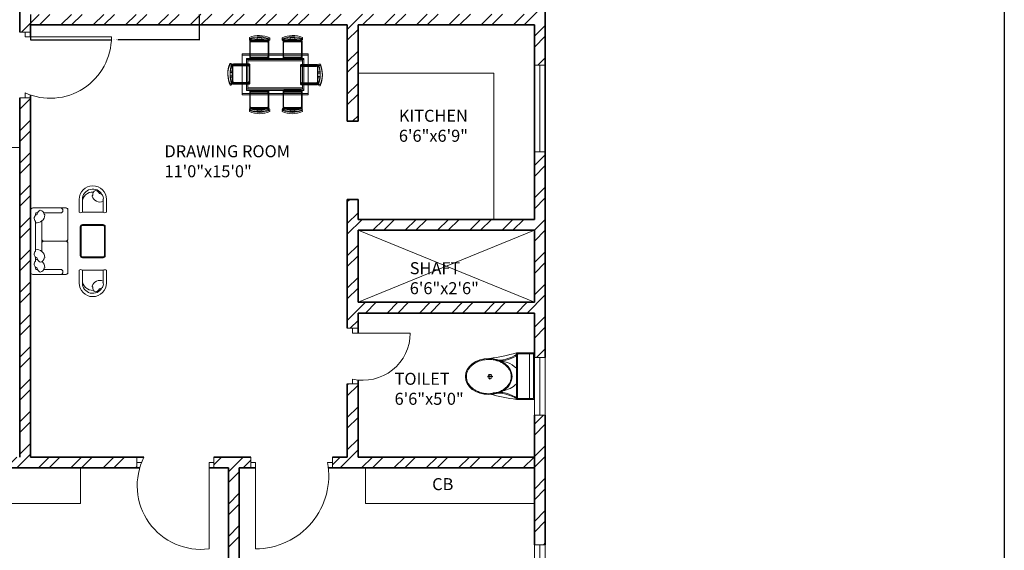
# Model space of a CAD drawing. Units: inches. Extents: x 2168 to 3056, y 1130 to 2629.
# Tile 6 of 42: x 2645 to 3056, y 1568 to 1789. Entities that reach past the tile are written whole.
import ezdxf

# ---------------------------------------------------------------- set-up
doc = ezdxf.new("R2010")
doc.units = ezdxf.units.IN
for name, color, linetype, lineweight in [('A-ANNO-DIMS', 2, 'Continuous', 18), ('A-ANNO-TEXT', 7, 'Continuous', 18), ('A-ANNO-TTLB', 7, 'Continuous', 25), ('A-AREA-IDEN', 7, 'Continuous', 18), ('A-DOOR', 21, 'Continuous', 18), ('A-FLOR-CASE', 71, 'Continuous', 18), ('A-FLOR-FIXT', 9, 'Continuous', 18), ('A-FLOR-OTLN', 7, 'Continuous', 18), ('A-FLOR-STRS', 71, 'Continuous', 18), ('A-FURN', 8, 'Continuous', 13), ('A-GLAZ', 201, 'Continuous', 18), ('A-WALL', 7, 'Continuous', 35)]:
    doc.layers.add(name, color=color, linetype=linetype, lineweight=lineweight)
doc.layers.add('A-WALL-PATT', color=143, linetype='Continuous', lineweight=13, true_color=0x7aafdf)
doc.styles.get("Standard").update_dxf_attribs({"font": 'arial.ttf'})
doc.dimstyles.get("Standard").update_dxf_attribs({"dimtxt": 0.18, "dimasz": 0.18, "dimexe": 0.18, "dimexo": 0.0625, "dimgap": 0.09, "dimtad": 0, "dimtih": 1, "dimtoh": 1, "dimdec": 4, "dimzin": 0, "dimdsep": 46, "dimtxsty": 'Standard', "dimcen": 0.09, "dimadec": 0, "dimazin": 0, "dimtfac": 1, "dimtdec": 4, "dimtofl": 0, "dimtmove": 0, "dimatfit": 3, "dimfxl": 1, "dimtolj": 1, "dimtzin": 0, "dimarcsym": 0})

# ---------------------------------------------------------------- blocks, each defined once
blk = doc.blocks.new('A$C31115884')
for p, q in [((283, 498), (223, 498)), ((258, 466), (258, 523)), ((0, 200), (0, 0)), ((520, 200), (0, 200)), ((10, 190), (10, 10)), ((510, 190), (10, 190)), ((510, 10), (510, 190)), ((520, 0), (520, 200)), ((510, 54), (0, 54)), ((10, 10), (510, 10)), ((0, 0), (520, 0))]:
    blk.add_line(p, q)
blk.add_circle((256, 496), 23.6)
for centre, radius, start, end in [((2778, -205), 2807, 165.4549, 171.7133), ((-295, 403), 365, 324.2091, 9.3499), ((-295, 403), 375, 324.2091, 9.3499), ((806, 403), 365, 170.6501, 215.7909), ((3237, 905), 2807, 188.2867, 194.5451), ((384, 406), 293, 190.2774, 224.1564), ((139, 406), 293, 315.8436, 2.6563), ((806, 403), 375, 179.2036, 215.7909)]:
    blk.add_arc(centre, radius, start, end)
blk.add_ellipse((256, 510), major_axis=(0, -261), ratio=0.772727)
blk.add_open_spline([(256, 259), (263, 259), (270, 260), (288, 262), (299, 265), (320, 273), (330, 278), (350, 291), (360, 299), (378, 316), (386, 326), (402, 347), (409, 358), (421, 383), (427, 395), (436, 422), (440, 436), (445, 465), (447, 480), (448, 509), (448, 524), (445, 553), (443, 568), (436, 596), (432, 610), (422, 636), (416, 649), (402, 672), (395, 683), (379, 703), (370, 712), (351, 728), (341, 735), (321, 746), (310, 751), (289, 757), (278, 759), (256, 761), (245, 761), (223, 757), (212, 754), (191, 746), (181, 741), (161, 728), (151, 720), (133, 703), (125, 693), (110, 672), (103, 660), (90, 636), (85, 623), (76, 596), (72, 582), (67, 553), (66, 538), (64, 509), (65, 494), (68, 465), (70, 450), (77, 422), (81, 408), (91, 382), (97, 370), (111, 346), (118, 335), (135, 316), (144, 307), (162, 291), (172, 284), (193, 273), (203, 269), (225, 262), (236, 260), (250, 259), (253, 259), (256, 259)], degree=3, knots=[0, 0, 0, 0, 0.110105, 0.110105, 0.285049, 0.285049, 0.459994, 0.459994, 0.634938, 0.634938, 0.809882, 0.809882, 0.984827, 0.984827, 1.159771, 1.159771, 1.334715, 1.334715, 1.50966, 1.50966, 1.684604, 1.684604, 1.859549, 1.859549, 2.034493, 2.034493, 2.209437, 2.209437, 2.384382, 2.384382, 2.559326, 2.559326, 2.73427, 2.73427, 2.909215, 2.909215, 3.084159, 3.084159, 3.259103, 3.259103, 3.434048, 3.434048, 3.608992, 3.608992, 3.783936, 3.783936, 3.958881, 3.958881, 4.133825, 4.133825, 4.30877, 4.30877, 4.483714, 4.483714, 4.658658, 4.658658, 4.833603, 4.833603, 5.008547, 5.008547, 5.183491, 5.183491, 5.358436, 5.358436, 5.53338, 5.53338, 5.708324, 5.708324, 5.883269, 5.883269, 6.058213, 6.058213, 6.233158, 6.233158, 6.283185, 6.283185, 6.283185, 6.283185])
blk = doc.blocks.new('A$C1352')
at = {"color": 0}
for points in [[(0.003, 0.053), (0.003, 0.553, -0.414214), (0.053, 0.603), (0.753, 0.603, -0.414214), (0.803, 0.553), (0.803, 0.053, -0.414214), (0.753, 0.003), (0.053, 0.003, -0.414214)], [(0.023, 0.053), (0.023, 0.553, -0.414214), (0.053, 0.583), (0.753, 0.583, -0.414214), (0.783, 0.553), (0.783, 0.053, -0.414214), (0.753, 0.023), (0.053, 0.023, -0.414214)]]:
    blk.add_lwpolyline(points, format="xyb", close=True, dxfattribs=at)
blk = doc.blocks.new('CHAIR-LOUNGE')
blk.add_line((10.04, 5.71), (10.04, 10.98))
at = {"ltscale": 0.03}
blk.add_lwpolyline([(10.04, 10.98, -0.369229), (11.42, 10.98), (11.42, 5.7, -1), (0, 5.72), (0, 10.99, -0.369229), (1.39, 10.99)], format="xyb", close=True, dxfattribs=at)
blk.add_lwpolyline([(9.55, 3.71, -0.785087), (1.38, 5.71), (1.39, 10.99)], format="xyb")
for centre, radius, start, end in [((5.71, 6.93), 4.33, 179.9461, 273.658), ((5.63, 4.23), 0.207, 150.6238, 293.7423), ((8.67, 3.43), 3.35, 67.0143, 164.2857), ((8.41, 5.02), 1.73, 272.9922, 34.1401), ((5.71, 5.71), 4.33, 358.8536, 359.9461), ((7.44, 3.63), 1.78, 166.6403, 249.4695), ((6.65, 3.91), 1.95, 274.9999, 341.3534)]:
    blk.add_arc(centre, radius, start, end)
blk = doc.blocks.new('TABLE-DINING')
for points in [[(0, 17.02), (27.45, 17.02), (27.45, 0.55), (0, 0.55)], [(0, 17.02), (27.45, 17.02), (27.45, 0.55), (0, 0.55)], [(0, 16.47), (27.45, 16.47), (27.45, 0), (0, 0)], [(0, 16.47), (27.45, 16.47), (27.45, 0), (0, 0)], [(1.83, 15.19), (25.62, 15.19), (25.62, 2.38), (1.83, 2.38)], [(1.83, 15.19), (25.62, 15.19), (25.62, 2.38), (1.83, 2.38)], [(1.83, 14.64), (25.62, 14.64), (25.62, 1.83), (1.83, 1.83)], [(1.83, 14.64), (25.62, 14.64), (25.62, 1.83), (1.83, 1.83)], [(2.38, 14.64), (25.07, 14.64), (25.07, 2.93), (2.38, 2.93)], [(2.38, 14.64), (25.07, 14.64), (25.07, 2.93), (2.38, 2.93)], [(2.38, 14.09), (25.07, 14.09), (25.07, 2.38), (2.38, 2.38)], [(2.38, 14.09), (25.07, 14.09), (25.07, 2.38), (2.38, 2.38)]]:
    blk.add_lwpolyline(points, close=True)
blk = doc.blocks.new('CUPBOARD-BEDROOM')
blk.add_lwpolyline([(0, 14.89), (70.36, 14.89), (70.36, 0), (0, 0)], close=True)
blk = doc.blocks.new('CHAIR-DINING-SIDE')
for points in [[(7.85, 2.38, 0.414214), (8.33, 2.86), (8.33, 9.24, 0.414214), (7.85, 9.73), (0.91, 9.73, 0.414214), (0.42, 9.24), (0.42, 2.86, 0.414214), (0.91, 2.38), (7.85, 2.38)], [(7.85, 2.38, 0.414214), (8.33, 2.86), (8.33, 9.24, 0.414214), (7.85, 9.73), (0.91, 9.73, 0.414214), (0.42, 9.24), (0.42, 2.86, 0.414214), (0.91, 2.38), (7.85, 2.38)], [(7.85, 1.83, 0.414214), (8.33, 2.31), (8.33, 8.69, 0.414214), (7.85, 9.18), (0.91, 9.18, 0.414214), (0.42, 8.69), (0.42, 2.31, 0.414214), (0.91, 1.83), (7.85, 1.83)], [(7.85, 1.83, 0.414214), (8.33, 2.31), (8.33, 8.69, 0.414214), (7.85, 9.18), (0.91, 9.18, 0.414214), (0.42, 8.69), (0.42, 2.31, 0.414214), (0.91, 1.83), (7.85, 1.83)], [(8.06, 2.08, -0.175809), (0.59, 2.13, 0.578392), (0.02, 1.51, 0.214524), (8.46, 1.4, 0.552014), (8.06, 2.08, -0.065079)], [(8.06, 2.08, -0.175809), (0.59, 2.13, 0.578392), (0.02, 1.51, 0.214524), (8.46, 1.4, 0.552014), (8.06, 2.08, -0.065079)], [(8.06, 1.53, -0.175809), (0.59, 1.58, 0.578392), (0.02, 0.96, 0.214524), (8.46, 0.85, 0.552014), (8.06, 1.53, -0.065079)], [(8.06, 1.53, -0.175809), (0.59, 1.58, 0.578392), (0.02, 0.96, 0.214524), (8.46, 0.85, 0.552014), (8.06, 1.53, -0.065079)], [(3.34, 2.38), (3.34, 1.5, -0.064759)], [(3.34, 2.38), (3.34, 1.5, -0.064759)], [(3.34, 1.83), (3.34, 0.95, -0.064759)], [(3.34, 1.83), (3.34, 0.95, -0.064759)]]:
    blk.add_lwpolyline(points, format="xyb")
for points in [[(7.84, 2.6), (1.13, 2.6, -0.414214), (0.64, 3.08), (0.64, 9.02, -0.414214), (1.13, 9.51), (7.84, 9.51, -0.512069), (8.11, 9.02), (8.11, 3.08, -0.512069)], [(7.84, 2.6), (1.13, 2.6, -0.414214), (0.64, 3.08), (0.64, 9.02, -0.414214), (1.13, 9.51), (7.84, 9.51, -0.512069), (8.11, 9.02), (8.11, 3.08, -0.512069)], [(7.84, 2.05), (1.13, 2.05, -0.414214), (0.64, 2.53), (0.64, 8.48, -0.414214), (1.13, 8.96), (7.84, 8.96, -0.512069), (8.11, 8.48), (8.11, 2.53, -0.512069)], [(7.84, 2.05), (1.13, 2.05, -0.414214), (0.64, 2.53), (0.64, 8.48, -0.414214), (1.13, 8.96), (7.84, 8.96, -0.512069), (8.11, 8.48), (8.11, 2.53, -0.512069)]]:
    blk.add_lwpolyline(points, format="xyb", close=True)
for points in [[(5.29, 1.48), (5.29, 2.38)], [(5.29, 1.48), (5.29, 2.38)], [(5.29, 0.93), (5.29, 1.83)], [(5.29, 0.93), (5.29, 1.83)]]:
    blk.add_lwpolyline(points)
blk = doc.blocks.new('CHAIR-DINING-END')
for points in [[(1.58, 1.14, -0.578392), (0.96, 0.57, -0.214524), (0.85, 9.01, -0.552014), (1.53, 8.61, 0.175809), (1.58, 1.14)], [(1.58, 1.14, -0.578392), (0.96, 0.57, -0.214524), (0.85, 9.01, -0.552014), (1.53, 8.61, 0.175809), (1.58, 1.14)], [(1.58, 0.59, -0.578392), (0.96, 0.02, -0.214524), (0.85, 8.46, -0.552014), (1.53, 8.06, 0.175809), (1.58, 0.59)], [(1.58, 0.59, -0.578392), (0.96, 0.02, -0.214524), (0.85, 8.46, -0.552014), (1.53, 8.06, 0.175809), (1.58, 0.59)], [(1.83, 8.39, -0.414214), (2.31, 8.88), (8.69, 8.88, -0.414214), (9.18, 8.39), (9.18, 1.45, -0.414214), (8.69, 0.97), (2.31, 0.97, -0.414214), (1.83, 1.45), (1.83, 8.39)], [(1.83, 8.39, -0.414214), (2.31, 8.88), (8.69, 8.88, -0.414214), (9.18, 8.39), (9.18, 1.45, -0.414214), (8.69, 0.97), (2.31, 0.97, -0.414214), (1.83, 1.45), (1.83, 8.39)], [(1.83, 7.85, -0.414214), (2.31, 8.33), (8.69, 8.33, -0.414214), (9.18, 7.85), (9.18, 0.91, -0.414214), (8.69, 0.42), (2.31, 0.42, -0.414214), (1.83, 0.91), (1.83, 7.85)], [(1.83, 7.85, -0.414214), (2.31, 8.33), (8.69, 8.33, -0.414214), (9.18, 7.85), (9.18, 0.91, -0.414214), (8.69, 0.42), (2.31, 0.42, -0.414214), (1.83, 0.91), (1.83, 7.85)], [(1.83, 3.89), (0.95, 3.89, 0.064759)], [(1.83, 3.89), (0.95, 3.89, 0.064759)], [(1.83, 3.34), (0.95, 3.34, 0.064759)], [(1.83, 3.34), (0.95, 3.34, 0.064759)]]:
    blk.add_lwpolyline(points, format="xyb")
for points in [[(2.05, 8.39), (2.05, 1.67, 0.414214), (2.53, 1.19), (8.48, 1.19, 0.414214), (8.96, 1.67), (8.96, 8.39, 0.512069), (8.48, 8.66), (2.53, 8.66, 0.512069)], [(2.05, 8.39), (2.05, 1.67, 0.414214), (2.53, 1.19), (8.48, 1.19, 0.414214), (8.96, 1.67), (8.96, 8.39, 0.512069), (8.48, 8.66), (2.53, 8.66, 0.512069)], [(2.05, 7.84), (2.05, 1.12, 0.414214), (2.53, 0.64), (8.48, 0.64, 0.414214), (8.96, 1.12), (8.96, 7.84, 0.512069), (8.48, 8.11), (2.53, 8.11, 0.512069)], [(2.05, 7.84), (2.05, 1.12, 0.414214), (2.53, 0.64), (8.48, 0.64, 0.414214), (8.96, 1.12), (8.96, 7.84, 0.512069), (8.48, 8.11), (2.53, 8.11, 0.512069)]]:
    blk.add_lwpolyline(points, format="xyb", close=True)
for points in [[(0.93, 5.84), (1.83, 5.84)], [(0.93, 5.83), (1.83, 5.83)], [(0.93, 5.29), (1.83, 5.29)], [(0.93, 5.29), (1.83, 5.29)]]:
    blk.add_lwpolyline(points)
blk = doc.blocks.new('WIN-24-OPPOSED-JAMBS')
for p, q in [((0, 4.5), (0, 0)), ((0, 4.5), (24, 4.5)), ((24, 2.25), (24, 4.5)), ((24, 4.5), (24, 0)), ((0, 0), (0, 2.25)), ((0, 2.25), (24, 2.25)), ((0, 0), (24, 0))]:
    blk.add_line(p, q)
blk = doc.blocks.new('WIN-60-OPPOSED-JAMBS')
for p, q in [((2.25, 60), (0, 60)), ((0, 60), (4.5, 60)), ((0, 60), (0, 0)), ((2.25, 0), (2.25, 60)), ((4.5, 60), (4.5, 0)), ((0, 0), (4.5, 0)), ((4.5, 0), (2.25, 0))]:
    blk.add_line(p, q)
blk = doc.blocks.new('*D18')
at = {"layer": 'A-ANNO-DIMS', "color": 0, "lineweight": -2, "transparency": 16777216}
for p, q in [((2649.8, 1791.2), (2649.8, 1780.53)), ((2720.15, 1791.2), (2720.15, 1780.53)), ((2649.98, 1780.71), (2683.7, 1780.71)), ((2719.97, 1780.71), (2686.25, 1780.71))]:
    blk.add_line(p, q, dxfattribs=at)
at = {"layer": 'A-ANNO-DIMS', "color": 0, "transparency": 16777216}
for points in [[(2649.98, 1780.74), (2649.98, 1780.68), (2649.8, 1780.71)], [(2719.97, 1780.74), (2719.97, 1780.68), (2720.15, 1780.71)]]:
    blk.add_solid(points, dxfattribs=at)
at = {"layer": 'Defpoints', "color": 0, "transparency": 16777216}
for p in [(2649.8, 1791.27), (2720.15, 1791.27), (2720.15, 1780.71)]:
    blk.add_point(p, dxfattribs=at)
at = {"layer": 'A-ANNO-DIMS', "color": 0, "transparency": 16777216, "insert": (2684.98, 1780.71), "char_height": 0.18, "attachment_point": 5}
blk.add_mtext('\\A1;CUPBOARD 70 TYP.', dxfattribs=at)

msp = doc.modelspace()

# ---------------------------------------------------------------- hatches: boundary and pattern name
at = {"layer": 'A-WALL-PATT'}
h = msp.add_hatch(dxfattribs=at)
h.set_pattern_fill('ANSI32', color=256)
h.paths.add_polyline_path([(2463.8, 2409.39), (2467.39, 2409.39), (2467.39, 2413.89), (2454.77, 2413.89), (2454.77, 2411.64), (2454.77, 2409.39), (2459.3, 2409.39), (2459.3, 2265.39), (2455.64, 2265.39), (2455.64, 2260.89), (2467.35, 2260.89), (2467.35, 2263.14), (2467.35, 2265.39), (2463.8, 2265.39)])
h.paths.add_polyline_path([(2431.6, 2413.89), (2409.65, 2413.89), (2409.65, 2409.39), (2431.6, 2409.39), (2431.6, 2411.64)])
h.paths.add_polyline_path([(2349.65, 2413.89), (2331.8, 2413.89), (2331.8, 2362.67), (2336.3, 2362.67), (2336.3, 2409.39), (2349.65, 2409.39), (2349.65, 2411.64)])
h.paths.add_polyline_path([(2634.15, 2411.64), (2634.15, 2413.89), (2562.29, 2413.89), (2562.29, 2409.39), (2595.8, 2409.39), (2595.8, 2280.31), (2595.83, 2280.31), (2595.83, 2265.39), (2499.91, 2265.39), (2499.91, 2260.89), (2550.8, 2260.89), (2550.8, 2117.31), (2555.3, 2117.31), (2555.3, 2168.08), (2571.93, 2168.08), (2571.93, 2176.89), (2559.8, 2176.89), (2559.8, 2256.39), (2640.8, 2256.39), (2640.8, 2176.89), (2626.43, 2176.89), (2626.43, 2168.08), (2645.3, 2168.08), (2645.3, 2116.64), (2649.8, 2116.64), (2649.8, 2260.89), (2691.25, 2260.89), (2691.25, 2263.14), (2691.25, 2265.39), (2670.65, 2265.39), (2670.65, 2265.36), (2600.3, 2265.36), (2600.3, 2280.26), (2600.3, 2409.39), (2634.15, 2409.39)])
h.paths.add_polyline_path([(2600.3, 2473.89), (2612.84, 2473.89), (2612.84, 2478.39), (2572.64, 2478.39), (2572.64, 2473.89), (2595.8, 2473.89), (2595.8, 2413.89), (2600.3, 2413.89)])
h.paths.add_polyline_path([(2535.8, 2473.89), (2548.64, 2473.89), (2548.64, 2478.39), (2531.4, 2478.39), (2531.4, 2413.89), (2521.6, 2413.89), (2521.6, 2409.39), (2539.24, 2409.39), (2539.24, 2411.64), (2539.24, 2413.89), (2535.8, 2413.89)])
h.paths.add_polyline_path([(2664.8, 2478.39), (2636.84, 2478.39), (2636.84, 2473.89), (2660.3, 2473.89), (2660.3, 2413.89), (2656.17, 2413.89), (2656.17, 2409.39), (2671.68, 2409.39), (2671.68, 2411.64), (2671.68, 2413.89), (2664.8, 2413.89)])
h.paths.add_polyline_path([(2705.94, 2413.89), (2695.68, 2413.89), (2695.68, 2409.39), (2705.94, 2409.39)])
h.paths.add_polyline_path([(2741.35, 2413.89), (2728.73, 2413.89), (2728.73, 2411.64), (2728.73, 2409.39), (2732.3, 2409.39), (2732.3, 2265.39), (2725.73, 2265.39), (2725.73, 2260.89), (2740.92, 2260.89), (2740.92, 2263.14), (2740.92, 2265.39), (2736.8, 2265.39), (2736.8, 2409.39), (2741.35, 2409.39)])
h.paths.add_polyline_path([(2785.65, 2413.89), (2764.55, 2413.89), (2764.49, 2409.39), (2785.65, 2409.39), (2785.65, 2411.64)])
h.paths.add_polyline_path([(2864.3, 2413.89), (2845.65, 2413.89), (2845.65, 2409.39), (2859.8, 2409.39), (2859.8, 2368.43), (2864.3, 2368.43)])
h.paths.add_polyline_path([(2864.3, 2308.43), (2862.05, 2308.43), (2859.8, 2308.43), (2859.8, 2265.39), (2774.48, 2265.39), (2774.48, 2263.14), (2774.48, 2260.89), (2781.8, 2260.89), (2781.8, 2226.65), (2786.3, 2226.65), (2786.3, 2260.89), (2859.8, 2260.89), (2859.8, 2241.35), (2864.3, 2241.35)])
h.paths.add_polyline_path([(2864.3, 2217.35), (2862.05, 2217.35), (2859.8, 2217.35), (2859.8, 2200.89), (2786.3, 2200.89), (2786.3, 2205.93), (2784.05, 2205.93), (2781.8, 2205.93), (2781.8, 2150.97), (2786.3, 2150.97), (2786.3, 2161.89), (2859.8, 2161.89), (2859.8, 2144.42), (2864.3, 2144.42)])
h.paths.add_polyline_path([(2859.8, 2196.39), (2859.8, 2166.39), (2786.3, 2166.39), (2786.3, 2196.39)], flags=16)
h.paths.add_polyline_path([(2864.3, 2108.42), (2862.05, 2108.42), (2859.8, 2108.42), (2859.8, 2080.89), (2786.3, 2080.89), (2786.3, 2111.99), (2781.8, 2111.99), (2781.8, 2080.89), (2649.8, 2080.89), (2649.8, 2086.04), (2647.55, 2086.04), (2645.3, 2086.04), (2645.3, 2071.74), (2649.8, 2071.74), (2649.8, 2076.39), (2781.8, 2076.39), (2781.8, 2041.79), (2786.3, 2041.79), (2786.3, 2076.39), (2859.8, 2076.39), (2859.8, 2058.58), (2864.3, 2058.58)])
h.paths.add_polyline_path([(2864.3, 2022.58), (2859.8, 2022.58), (2859.8, 1992.39), (2786.3, 1992.39), (2786.3, 1999.57), (2781.8, 1999.57), (2781.8, 1848.09), (2784.05, 1848.09), (2786.3, 1848.09), (2786.3, 1851.39), (2859.8, 1851.39), (2859.8, 1838.26), (2864.3, 1838.26)], flags=17)
h.paths.add_polyline_path([(2859.8, 1987.89), (2859.8, 1855.89), (2786.3, 1855.89), (2786.3, 1987.89)], flags=16)
h.paths.add_polyline_path([(2823.05, 1987.89), (2841.42, 1921.89), (2823.05, 1855.89)], flags=0)
h.paths.add_polyline_path([(2864.3, 1814.26), (2859.8, 1814.26), (2859.8, 1791.39), (2786.3, 1791.39), (2786.3, 1825.66), (2784.05, 1825.66), (2781.8, 1825.66), (2781.8, 1791.39), (2720.15, 1791.39), (2720.15, 1791.27), (2649.8, 1791.27), (2649.8, 1806.16), (2649.8, 2038.98), (2647.55, 2038.98), (2645.3, 2038.98), (2645.3, 1783.93), (2649.8, 1783.93), (2649.8, 1786.89), (2781.8, 1786.89), (2781.8, 1746.79), (2786.3, 1746.79), (2786.3, 1786.89), (2859.8, 1786.89), (2859.8, 1770.08), (2864.3, 1770.08)])
h.paths.add_polyline_path([(2864.3, 1734.08), (2862.05, 1734.08), (2859.8, 1734.08), (2859.8, 1705.89), (2786.3, 1705.89), (2786.3, 1714.17), (2781.8, 1714.17), (2781.8, 1660.53), (2786.3, 1660.53), (2786.3, 1666.89), (2859.8, 1666.89), (2859.8, 1648.34), (2864.3, 1648.34)])
h.paths.add_polyline_path([(2786.3, 1701.39), (2859.8, 1701.39), (2859.8, 1671.39), (2786.3, 1671.39)], flags=16)
h.paths.add_polyline_path([(2649.8, 1756.58), (2647.55, 1756.58), (2645.3, 1756.58), (2645.3, 1606.89), (2555.3, 1606.89), (2555.3, 1749.51), (2553.05, 1749.51), (2550.8, 1749.51), (2550.8, 1606.89), (2503.01, 1606.89), (2503.01, 1604.64), (2503.01, 1602.39), (2595.8, 1602.39), (2595.85, 1602.39), (2595.85, 1587.5), (2595.8, 1458.39), (2561.5, 1458.39), (2561.5, 1456.14), (2561.5, 1453.89), (2595.8, 1453.89), (2595.8, 1381.89), (2573.44, 1381.89), (2573.44, 1377.39), (2613.01, 1377.39), (2613.01, 1379.64), (2613.01, 1381.89), (2600.3, 1381.89), (2600.3, 1453.89), (2634.33, 1453.89), (2634.33, 1458.39), (2600.3, 1458.39), (2600.3, 1602.39), (2670.65, 1602.39), (2694.09, 1602.39), (2694.09, 1606.89), (2649.8, 1606.89)])
h.paths.add_polyline_path([(2736.8, 1602.39), (2741.56, 1602.39), (2741.56, 1606.89), (2726.2, 1606.89), (2726.2, 1604.64), (2726.2, 1602.39), (2732.3, 1602.39), (2732.3, 1458.39), (2727.9, 1458.39), (2727.9, 1453.89), (2740.82, 1453.89), (2740.82, 1456.14), (2740.82, 1458.39), (2736.8, 1458.39)])
h.paths.add_polyline_path([(2859.8, 1606.89), (2786.3, 1606.89), (2786.3, 1637.33), (2784.05, 1637.33), (2781.8, 1637.33), (2781.8, 1606.89), (2775.61, 1606.89), (2775.61, 1602.39), (2859.8, 1602.39)])
h.paths.add_polyline_path([(2864.3, 1624.34), (2862.05, 1624.34), (2859.8, 1624.34), (2859.8, 1570.39), (2864.3, 1570.39)])
h.paths.add_polyline_path([(2864.3, 1510.39), (2862.05, 1510.39), (2859.8, 1510.39), (2859.8, 1458.39), (2846.73, 1458.39), (2846.73, 1456.14), (2846.73, 1453.89), (2864.3, 1453.89)])
h.paths.add_polyline_path([(2786.73, 1458.39), (2765.44, 1458.39), (2765.44, 1453.89), (2786.73, 1453.89)])
h.paths.add_polyline_path([(2706, 1458.39), (2695.36, 1458.39), (2695.36, 1453.89), (2706, 1453.89), (2706, 1456.14)])
h.paths.add_polyline_path([(2671.36, 1456.14), (2671.36, 1458.39), (2655.99, 1458.39), (2655.99, 1456.14), (2655.99, 1453.89), (2660.3, 1453.89), (2660.3, 1381.89), (2637.01, 1381.89), (2637.01, 1377.39), (2664.8, 1377.39), (2664.8, 1453.89), (2671.36, 1453.89)], flags=17)
h.paths.add_polyline_path([(2539.83, 1458.39), (2520.24, 1458.39), (2520.24, 1453.89), (2531.3, 1453.89), (2531.3, 1377.39), (2546.45, 1377.39), (2546.45, 1379.64), (2546.45, 1381.89), (2535.8, 1381.89), (2535.8, 1453.89), (2539.83, 1453.89)], flags=17)
h.paths.add_polyline_path([(2496.24, 1458.39), (2489.13, 1458.39), (2489.13, 1453.89), (2496.24, 1453.89), (2496.24, 1456.14)])
h.paths.add_polyline_path([(2467.43, 1456.14), (2467.43, 1458.39), (2463.8, 1458.39), (2463.8, 1602.39), (2468.24, 1602.39), (2468.24, 1605.7), (2468.24, 1606.89), (2454.6, 1606.89), (2454.6, 1602.39), (2459.3, 1602.39), (2459.3, 1458.39), (2454.24, 1458.39), (2454.24, 1453.89), (2467.43, 1453.89)])
h.paths.add_polyline_path([(2431.6, 1456.14), (2431.6, 1458.39), (2411.39, 1458.39), (2411.39, 1453.89), (2431.6, 1453.89)])
h.paths.add_polyline_path([(2351.39, 1458.39), (2336.3, 1458.39), (2336.3, 1490.69), (2334.05, 1490.69), (2331.8, 1490.69), (2331.8, 1453.89), (2351.39, 1453.89), (2351.39, 1456.14)])
h.paths.add_polyline_path([(2336.3, 1629.7), (2331.8, 1629.7), (2331.8, 1552.32), (2336.3, 1552.32), (2336.3, 1602.39), (2406.65, 1602.39), (2423.47, 1602.39), (2423.47, 1606.89), (2418.8, 1606.89), (2418.8, 1643.68), (2416.55, 1643.68), (2414.3, 1643.68), (2414.3, 1606.89), (2336.3, 1606.89)])
h.paths.add_polyline_path([(2418.8, 1714.38), (2414.3, 1714.38), (2414.3, 1705.89), (2336.3, 1705.89), (2336.3, 1731.32), (2334.05, 1731.32), (2331.8, 1731.32), (2331.8, 1653.7), (2334.05, 1653.7), (2336.3, 1653.7), (2336.3, 1666.89), (2414.3, 1666.89), (2414.3, 1663.59), (2418.8, 1663.59)])
h.paths.add_polyline_path([(2336.3, 1701.39), (2414.3, 1701.39), (2414.3, 1671.39), (2336.3, 1671.39)], flags=16)
h.paths.add_polyline_path([(2555.3, 2040.06), (2550.8, 2040.06), (2550.8, 1791.39), (2550.56, 1791.2), (2480.2, 1791.2), (2418.8, 1791.39), (2418.8, 1825.45), (2416.55, 1825.45), (2414.3, 1825.45), (2414.3, 1791.39), (2336.3, 1791.39), (2336.3, 1806.41), (2331.8, 1806.41), (2331.8, 1767.32), (2336.3, 1767.32), (2336.3, 1786.89), (2414.3, 1786.89), (2414.3, 1745.46), (2418.8, 1745.46), (2418.8, 1786.89), (2550.8, 1786.89), (2550.8, 1783.01), (2555.3, 1783.01)])
h.paths.add_polyline_path([(2418.8, 1923.39), (2423.21, 1923.39), (2423.21, 1925.64), (2423.21, 1927.89), (2418.8, 1927.89), (2418.8, 2000.05), (2414.3, 2000.05), (2414.3, 1992.39), (2336.3, 1992.39), (2336.3, 1987.89), (2414.3, 1987.89), (2414.3, 1855.89), (2336.3, 1855.89), (2336.3, 1851.39), (2414.3, 1851.39), (2414.3, 1846.76), (2418.8, 1846.76)], flags=17)
h.paths.add_polyline_path([(2336.3, 2019.29), (2334.05, 2019.29), (2331.8, 2019.29), (2331.8, 1830.41), (2336.3, 1830.41)], flags=17)
h.paths.add_polyline_path([(2550.8, 1927.89), (2453.54, 1927.89), (2453.54, 1925.64), (2453.54, 1923.39), (2550.8, 1923.39)], flags=17)
h.paths.add_polyline_path([(2744.99, 1927.89), (2649.8, 1927.89), (2649.8, 1923.39), (2744.99, 1923.39), (2744.99, 1925.64)], flags=17)
h.paths.add_polyline_path([(2555.3, 2086.46), (2553.05, 2086.46), (2550.8, 2086.46), (2550.8, 2080.89), (2418.8, 2080.89), (2336.3, 2080.89), (2336.3, 2115.4), (2334.05, 2115.4), (2331.8, 2115.4), (2331.8, 2055.29), (2336.3, 2055.29), (2336.3, 2076.39), (2550.8, 2076.39), (2550.8, 2071.54), (2555.3, 2071.54)])
h.paths.add_polyline_path([(2418.8, 2121.39), (2414.3, 2121.39), (2414.3, 2080.89), (2418.8, 2080.89)])
h.paths.add_polyline_path([(2418.8, 2076.39), (2414.3, 2076.39), (2414.3, 2035.12), (2418.8, 2035.12)])
h.paths.add_polyline_path([(2422.87, 2263.14), (2422.87, 2265.39), (2406.65, 2265.39), (2406.65, 2265.36), (2336.3, 2265.36), (2336.3, 2280.25), (2336.3, 2302.67), (2334.05, 2302.67), (2331.8, 2302.67), (2331.8, 2246.85), (2336.3, 2246.85), (2336.3, 2260.89), (2414.3, 2260.89), (2414.3, 2224), (2418.8, 2224), (2418.8, 2260.89), (2422.87, 2260.89)])
h.paths.add_polyline_path([(2418.8, 2204.78), (2416.55, 2204.78), (2414.3, 2204.78), (2414.3, 2200.89), (2336.3, 2200.89), (2336.3, 2220.85), (2331.8, 2220.85), (2331.8, 2151.4), (2336.3, 2151.4), (2336.3, 2161.89), (2414.3, 2161.89), (2414.3, 2153.73), (2418.8, 2153.73)])
h.paths.add_polyline_path([(2414.3, 2196.39), (2414.3, 2166.39), (2336.3, 2166.39), (2336.3, 2196.39)], flags=16)
h.paths.add_polyline_path([(2375.3, 2181.39), (2336.3, 2166.39), (2336.3, 2196.39)], flags=0)
h.paths.add_polyline_path([(2809.6, 2172.34), (2838.8, 2172.34), (2838.8, 2191), (2809.6, 2191)], flags=8)
h.paths.add_polyline_path([(2849.75, 1919.59), (2849.75, 1952.67), (2831.09, 1952.67), (2831.09, 1919.59)], flags=8)
h.paths.add_polyline_path([(2808.87, 1901.97), (2808.87, 1937.85), (2790.15, 1937.85), (2790.15, 1901.97)], flags=8)
h.paths.add_polyline_path([(2806.28, 1671.9), (2835.49, 1671.9), (2835.49, 1690.55), (2806.28, 1690.55)], flags=8)
h.paths.add_polyline_path([(2353.19, 1676.55), (2382.39, 1676.55), (2382.39, 1695.21), (2353.19, 1695.21)], flags=8)
h.paths.add_polyline_path([(2360.08, 1832.31), (2389.24, 1832.31), (2389.24, 1850.97), (2360.08, 1850.97)], flags=25)
h.paths.add_polyline_path([(2354.82, 2167.82), (2384.03, 2167.82), (2384.03, 2186.48), (2354.82, 2186.48)], flags=8)

# ---------------------------------------------------------------- linework, layer by layer
at = {"layer": 'A-ANNO-TTLB'}
msp.add_lwpolyline([(2168.16, 2629.19), (3055.63, 2629.19), (3055.63, 1130.19), (2168.16, 1130.19)], close=True, dxfattribs=at)
at = {"layer": 'A-DOOR'}
for p, q in [((2645.3, 1783.93), (2649.8, 1783.93)), ((2649.8, 1783.93), (2647.55, 1783.93)), ((2647.55, 1783.93), (2647.55, 1781.93)), ((2647.55, 1781.93), (2683.55, 1781.93)), ((2645.3, 1756.58), (2649.8, 1756.58)), ((2647.55, 1756.58), (2647.55, 1758.58)), ((2649.8, 1756.58), (2647.55, 1756.58)), ((2781.8, 1660.53), (2786.3, 1660.53)), ((2786.3, 1660.53), (2784.05, 1660.53)), ((2784.05, 1660.53), (2784.05, 1658.53)), ((2784.05, 1658.53), (2808.05, 1658.53)), ((2781.8, 1637.33), (2786.3, 1637.33)), ((2784.05, 1637.33), (2784.05, 1639.33)), ((2786.3, 1637.33), (2784.05, 1637.33)), ((2694.09, 1602.39), (2694.09, 1606.89)), ((2694.09, 1606.89), (2694.09, 1604.64)), ((2694.09, 1604.64), (2696.09, 1604.64)), ((2726.2, 1604.64), (2724.2, 1604.64)), ((2724.2, 1604.64), (2724.2, 1568.64)), ((2726.2, 1602.39), (2726.2, 1606.89)), ((2726.2, 1606.89), (2726.2, 1604.64)), ((2741.56, 1602.39), (2741.56, 1606.89)), ((2741.56, 1606.89), (2741.56, 1604.64)), ((2741.56, 1604.64), (2743.56, 1604.64)), ((2743.56, 1604.64), (2743.56, 1568.64)), ((2775.61, 1604.64), (2773.61, 1604.64)), ((2775.61, 1606.89), (2775.61, 1602.39)), ((2775.61, 1602.39), (2775.61, 1604.64))]:
    msp.add_line(p, q, dxfattribs=at)
for centre, radius, start, end in [((2657.97, 1781.93), 25.57, 245.9356, 360), ((2788.37, 1658.53), 19.67, 257.2991, 0), ((2720.82, 1594.97), 26.55, 153.3212, 277.3252), ((2743.56, 1599.18), 30.54, 270, 10.2947)]:
    msp.add_arc(centre, radius, start, end, dxfattribs=at)
at = {"layer": 'A-FLOR-CASE'}
for p, q in [((2786.3, 1766.84), (2842.96, 1766.84)), ((2842.96, 1766.84), (2842.96, 1705.89))]:
    msp.add_line(p, q, dxfattribs=at)
at = {"layer": 'A-FLOR-OTLN'}
for p, q in [((2786.3, 1671.39), (2859.8, 1701.39)), ((2786.3, 1701.39), (2859.8, 1671.39))]:
    msp.add_line(p, q, dxfattribs=at)
at = {"layer": 'A-FLOR-STRS'}
msp.add_line((2555.3, 1735.84), (2645.3, 1735.84), dxfattribs=at)
at = {"layer": 'A-FURN'}
for p, q in [((2651.87, 1708.23), (2651.87, 1707.59)), ((2652.7, 1708.57), (2652.22, 1708.57)), ((2662.25, 1708.57), (2655.33, 1708.57)), ((2651.87, 1705.09), (2651.87, 1692.68)), ((2651.87, 1689.54), (2651.87, 1690.18)), ((2651.87, 1690.18), (2651.87, 1688.52)), ((2651.87, 1685.39), (2651.87, 1686.03)), ((2652.7, 1685.04), (2652.22, 1685.04)), ((2655.33, 1685.04), (2662.25, 1685.04))]:
    msp.add_line(p, q, dxfattribs=at)
for points in [[(2741.45, 1780.97, -0.175809), (2748.92, 1780.91, 0.578392), (2749.49, 1781.53, 0.214524), (2741.05, 1781.65, 0.552014), (2741.45, 1780.97, -0.065079)], [(2741.45, 1780.97, -0.175809), (2748.92, 1780.91, 0.578392), (2749.49, 1781.53, 0.214524), (2741.05, 1781.65, 0.552014), (2741.45, 1780.97, -0.065079)], [(2741.45, 1780.42, -0.175809), (2748.92, 1780.36, 0.578392), (2749.49, 1780.98, 0.214524), (2741.05, 1781.1, 0.552014), (2741.45, 1780.42, -0.065079)], [(2741.45, 1780.42, -0.175809), (2748.92, 1780.36, 0.578392), (2749.49, 1780.98, 0.214524), (2741.05, 1781.1, 0.552014), (2741.45, 1780.42, -0.065079)], [(2746.17, 1780.67), (2746.17, 1781.55, -0.064759)], [(2746.17, 1780.67), (2746.17, 1781.54, -0.064759)], [(2746.17, 1780.12), (2746.17, 1781, -0.064759)], [(2746.17, 1780.12), (2746.17, 1781, -0.064759)], [(2755.22, 1780.91, -0.578392), (2754.65, 1781.53, -0.214524), (2763.09, 1781.65, -0.552014), (2762.69, 1780.97, 0.175809), (2755.22, 1780.91)], [(2755.22, 1780.91, -0.578392), (2754.65, 1781.53, -0.214524), (2763.09, 1781.65, -0.552014), (2762.69, 1780.97, 0.175809), (2755.22, 1780.91)], [(2755.22, 1780.36, -0.578392), (2754.65, 1780.98, -0.214524), (2763.09, 1781.1, -0.552014), (2762.69, 1780.42, 0.175809), (2755.22, 1780.36)], [(2755.22, 1780.36, -0.578392), (2754.65, 1780.98, -0.214524), (2763.09, 1781.1, -0.552014), (2762.69, 1780.42, 0.175809), (2755.22, 1780.36)], [(2757.97, 1780.67), (2757.97, 1781.55, 0.064759)], [(2757.97, 1780.67), (2757.97, 1781.54, 0.064759)], [(2757.97, 1780.12), (2757.97, 1781, 0.064759)], [(2757.97, 1780.12), (2757.97, 1781, 0.064759)], [(2748.61, 1780.67), (2741.67, 1780.67, 0.414214), (2741.18, 1780.18), (2741.18, 1773.8, 0.414214), (2741.67, 1773.32), (2748.61, 1773.32, 0.414214), (2749.09, 1773.8), (2749.09, 1780.18, 0.414214), (2748.61, 1780.67)], [(2748.61, 1780.67), (2741.67, 1780.67, 0.414214), (2741.18, 1780.18), (2741.18, 1773.8, 0.414214), (2741.67, 1773.32), (2748.61, 1773.32, 0.414214), (2749.09, 1773.8), (2749.09, 1780.18, 0.414214), (2748.61, 1780.67)], [(2748.61, 1780.12), (2741.67, 1780.12, 0.414214), (2741.18, 1779.63), (2741.18, 1773.25, 0.414214), (2741.67, 1772.77), (2748.61, 1772.77, 0.414214), (2749.09, 1773.25), (2749.09, 1779.63, 0.414214), (2748.61, 1780.12)], [(2748.61, 1780.12), (2741.67, 1780.12, 0.414214), (2741.18, 1779.63), (2741.18, 1773.25, 0.414214), (2741.67, 1772.77), (2748.61, 1772.77, 0.414214), (2749.09, 1773.25), (2749.09, 1779.63, 0.414214), (2748.61, 1780.12)], [(2762.47, 1780.67, -0.414214), (2762.96, 1780.18), (2762.96, 1773.8, -0.414214), (2762.47, 1773.32), (2755.53, 1773.32, -0.414214), (2755.05, 1773.8), (2755.05, 1780.18, -0.414214), (2755.53, 1780.67), (2762.47, 1780.67)], [(2762.47, 1780.67, -0.414214), (2762.96, 1780.18), (2762.96, 1773.8, -0.414214), (2762.47, 1773.32), (2755.53, 1773.32, -0.414214), (2755.05, 1773.8), (2755.05, 1780.18, -0.414214), (2755.53, 1780.67), (2762.47, 1780.67)], [(2762.47, 1780.12, -0.414214), (2762.96, 1779.63), (2762.96, 1773.25, -0.414214), (2762.47, 1772.77), (2755.53, 1772.77, -0.414214), (2755.05, 1773.25), (2755.05, 1779.63, -0.414214), (2755.53, 1780.12), (2762.47, 1780.12)], [(2762.47, 1780.12, -0.414214), (2762.96, 1779.63), (2762.96, 1773.25, -0.414214), (2762.47, 1772.77), (2755.53, 1772.77, -0.414214), (2755.05, 1773.25), (2755.05, 1779.63, -0.414214), (2755.53, 1780.12), (2762.47, 1780.12)], [(2733.63, 1762.92, -0.578392), (2733.01, 1762.35, -0.214524), (2732.89, 1770.79, -0.552014), (2733.57, 1770.39, 0.175809), (2733.63, 1762.92)], [(2733.63, 1762.92, -0.578392), (2733.01, 1762.35, -0.214524), (2732.89, 1770.79, -0.552014), (2733.57, 1770.39, 0.175809), (2733.63, 1762.92)], [(2733.63, 1762.37, -0.578392), (2733.01, 1761.8, -0.214524), (2732.89, 1770.24, -0.552014), (2733.57, 1769.84, 0.175809), (2733.63, 1762.37)], [(2733.63, 1762.37, -0.578392), (2733.01, 1761.8, -0.214524), (2732.89, 1770.24, -0.552014), (2733.57, 1769.84, 0.175809), (2733.63, 1762.37)], [(2733.87, 1770.17, -0.414214), (2734.36, 1770.66), (2740.74, 1770.66, -0.414214), (2741.22, 1770.17), (2741.22, 1763.23, -0.414214), (2740.74, 1762.75), (2734.36, 1762.75, -0.414214), (2733.87, 1763.23), (2733.87, 1770.17)], [(2733.87, 1770.17, -0.414214), (2734.36, 1770.66), (2740.74, 1770.66, -0.414214), (2741.22, 1770.17), (2741.22, 1763.23, -0.414214), (2740.74, 1762.75), (2734.36, 1762.75, -0.414214), (2733.87, 1763.23), (2733.87, 1770.17)], [(2733.87, 1769.62, -0.414214), (2734.36, 1770.11), (2740.74, 1770.11, -0.414214), (2741.22, 1769.62), (2741.22, 1762.68, -0.414214), (2740.74, 1762.2), (2734.36, 1762.2, -0.414214), (2733.87, 1762.68), (2733.87, 1769.62)], [(2733.87, 1769.62, -0.414214), (2734.36, 1770.11), (2740.74, 1770.11, -0.414214), (2741.22, 1769.62), (2741.22, 1762.68, -0.414214), (2740.74, 1762.2), (2734.36, 1762.2, -0.414214), (2733.87, 1762.68), (2733.87, 1769.62)], [(2733.87, 1765.67), (2732.99, 1765.67, 0.064759)], [(2733.87, 1765.67), (2732.99, 1765.67, 0.064759)], [(2733.87, 1765.12), (2732.99, 1765.12, 0.064759)], [(2733.87, 1765.12), (2732.99, 1765.12, 0.064759)], [(2748.61, 1752.3), (2741.67, 1752.3, -0.414214), (2741.18, 1752.79), (2741.18, 1759.17, -0.414214), (2741.67, 1759.65), (2748.61, 1759.65, -0.414214), (2749.09, 1759.17), (2749.09, 1752.79, -0.414214), (2748.61, 1752.3)], [(2748.61, 1752.3), (2741.67, 1752.3, -0.414214), (2741.18, 1752.79), (2741.18, 1759.17, -0.414214), (2741.67, 1759.65), (2748.61, 1759.65, -0.414214), (2749.09, 1759.17), (2749.09, 1752.79, -0.414214), (2748.61, 1752.3)], [(2748.61, 1751.75), (2741.67, 1751.75, -0.414214), (2741.18, 1752.24), (2741.18, 1758.62, -0.414214), (2741.67, 1759.11), (2748.61, 1759.11, -0.414214), (2749.09, 1758.62), (2749.09, 1752.24, -0.414214), (2748.61, 1751.75)], [(2748.61, 1751.75), (2741.67, 1751.75, -0.414214), (2741.18, 1752.24), (2741.18, 1758.62, -0.414214), (2741.67, 1759.1), (2748.61, 1759.1, -0.414214), (2749.09, 1758.62), (2749.09, 1752.24, -0.414214), (2748.61, 1751.75)], [(2746.17, 1752.3), (2746.17, 1751.42, 0.064759)], [(2746.17, 1752.3), (2746.17, 1751.42, 0.064759)], [(2748.92, 1752.06, -0.578392), (2749.49, 1751.44, -0.214524), (2741.05, 1751.32, -0.552014), (2741.45, 1752, 0.175809), (2748.92, 1752.06)], [(2748.92, 1752.06, -0.578392), (2749.49, 1751.44, -0.214524), (2741.05, 1751.32, -0.552014), (2741.45, 1752, 0.175809), (2748.92, 1752.06)], [(2748.92, 1751.51, -0.578392), (2749.49, 1750.89, -0.214524), (2741.05, 1750.77, -0.552014), (2741.45, 1751.45, 0.175809), (2748.92, 1751.51)], [(2748.92, 1751.51, -0.578392), (2749.49, 1750.89, -0.214524), (2741.05, 1750.77, -0.552014), (2741.45, 1751.45, 0.175809), (2748.92, 1751.51)], [(2746.17, 1751.75), (2746.17, 1750.88, 0.064759)], [(2746.17, 1751.75), (2746.17, 1750.87, 0.064759)], [(2654.55, 1704.64), (2654.55, 1697.67, 0.414214), (2655.42, 1696.81), (2664.5, 1696.81, 0.414214), (2665.37, 1697.67), (2665.37, 1709.79, 0.414214), (2664.5, 1710.65)], [(2654.55, 1692.54), (2654.55, 1695.94, -0.414214), (2655.42, 1696.81), (2664.5, 1696.81, -0.414214), (2665.37, 1695.94), (2665.37, 1683.83, -0.414214), (2664.5, 1682.97)]]:
    msp.add_lwpolyline(points, format="xyb", dxfattribs=at)
for points in [[(2744.23, 1781.56), (2744.23, 1780.67)], [(2744.23, 1781.56), (2744.23, 1780.67)], [(2744.23, 1781.01), (2744.23, 1780.12)], [(2744.23, 1781.01), (2744.23, 1780.12)], [(2759.91, 1781.56), (2759.91, 1780.67)], [(2759.91, 1781.56), (2759.91, 1780.67)], [(2759.91, 1781.01), (2759.91, 1780.12)], [(2759.91, 1781.01), (2759.91, 1780.12)], [(2732.98, 1767.61), (2733.87, 1767.61)], [(2732.98, 1767.61), (2733.87, 1767.61)], [(2732.98, 1767.06), (2733.87, 1767.06)], [(2732.98, 1767.06), (2733.87, 1767.06)], [(2744.23, 1751.41), (2744.23, 1752.3)], [(2744.23, 1751.41), (2744.23, 1752.3)], [(2744.23, 1750.86), (2744.23, 1751.75)], [(2744.23, 1750.86), (2744.23, 1751.75)], [(2654.55, 1692.54), (2654.55, 1705.23)]]:
    msp.add_lwpolyline(points, dxfattribs=at)
for points in [[(2741.67, 1780.45), (2748.39, 1780.45, -0.414214), (2748.87, 1779.96), (2748.87, 1774.02, -0.414214), (2748.39, 1773.53), (2741.67, 1773.53, -0.512069), (2741.4, 1774.02), (2741.4, 1779.96, -0.512069)], [(2741.67, 1780.45), (2748.39, 1780.45, -0.414214), (2748.87, 1779.96), (2748.87, 1774.02, -0.414214), (2748.39, 1773.53), (2741.67, 1773.53, -0.512069), (2741.4, 1774.02), (2741.4, 1779.96, -0.512069)], [(2741.67, 1779.9), (2748.39, 1779.9, -0.414214), (2748.87, 1779.41), (2748.87, 1773.47, -0.414214), (2748.39, 1772.99), (2741.67, 1772.99, -0.512069), (2741.4, 1773.47), (2741.4, 1779.41, -0.512069)], [(2741.67, 1779.9), (2748.39, 1779.9, -0.414214), (2748.87, 1779.41), (2748.87, 1773.47, -0.414214), (2748.39, 1772.98), (2741.67, 1772.98, -0.512069), (2741.4, 1773.47), (2741.4, 1779.41, -0.512069)], [(2762.47, 1780.45), (2755.75, 1780.45, 0.414214), (2755.27, 1779.96), (2755.27, 1774.02, 0.414214), (2755.75, 1773.53), (2762.47, 1773.53, 0.512069), (2762.74, 1774.02), (2762.74, 1779.96, 0.512069)], [(2762.47, 1780.45), (2755.75, 1780.45, 0.414214), (2755.27, 1779.96), (2755.27, 1774.02, 0.414214), (2755.75, 1773.53), (2762.47, 1773.53, 0.512069), (2762.74, 1774.02), (2762.74, 1779.96, 0.512069)], [(2762.47, 1779.9), (2755.75, 1779.9, 0.414214), (2755.27, 1779.41), (2755.27, 1773.47, 0.414214), (2755.75, 1772.99), (2762.47, 1772.99, 0.512069), (2762.74, 1773.47), (2762.74, 1779.41, 0.512069)], [(2762.47, 1779.9), (2755.75, 1779.9, 0.414214), (2755.27, 1779.41), (2755.27, 1773.47, 0.414214), (2755.75, 1772.98), (2762.47, 1772.98, 0.512069), (2762.74, 1773.47), (2762.74, 1779.41, 0.512069)], [(2734.09, 1770.17), (2734.09, 1763.45, 0.414214), (2734.58, 1762.97), (2740.52, 1762.97, 0.414214), (2741, 1763.45), (2741, 1770.17, 0.512069), (2740.52, 1770.44), (2734.58, 1770.44, 0.512069)], [(2734.09, 1770.17), (2734.09, 1763.45, 0.414214), (2734.58, 1762.97), (2740.52, 1762.97, 0.414214), (2741, 1763.45), (2741, 1770.17, 0.512069), (2740.52, 1770.44), (2734.58, 1770.44, 0.512069)], [(2734.09, 1769.62), (2734.09, 1762.9, 0.414214), (2734.58, 1762.42), (2740.52, 1762.42, 0.414214), (2741, 1762.9), (2741, 1769.62, 0.512069), (2740.52, 1769.89), (2734.58, 1769.89, 0.512069)], [(2734.09, 1769.62), (2734.09, 1762.9, 0.414214), (2734.58, 1762.42), (2740.52, 1762.42, 0.414214), (2741, 1762.9), (2741, 1769.62, 0.512069), (2740.52, 1769.89), (2734.58, 1769.89, 0.512069)], [(2741.67, 1752.52), (2748.39, 1752.52, 0.414214), (2748.87, 1753.01), (2748.87, 1758.95, 0.414214), (2748.39, 1759.44), (2741.67, 1759.44, 0.512069), (2741.4, 1758.95), (2741.4, 1753.01, 0.512069)], [(2741.67, 1752.52), (2748.39, 1752.52, 0.414214), (2748.87, 1753.01), (2748.87, 1758.95, 0.414214), (2748.39, 1759.43), (2741.67, 1759.43, 0.512069), (2741.4, 1758.95), (2741.4, 1753.01, 0.512069)], [(2741.67, 1751.97), (2748.39, 1751.97, 0.414214), (2748.87, 1752.46), (2748.87, 1758.4, 0.414214), (2748.39, 1758.89), (2741.67, 1758.89, 0.512069), (2741.4, 1758.4), (2741.4, 1752.46, 0.512069)], [(2741.67, 1751.97), (2748.39, 1751.97, 0.414214), (2748.87, 1752.46), (2748.87, 1758.4, 0.414214), (2748.39, 1758.89), (2741.67, 1758.89, 0.512069), (2741.4, 1758.4), (2741.4, 1752.46, 0.512069)]]:
    msp.add_lwpolyline(points, format="xyb", close=True, dxfattribs=at)
at = {"layer": 'A-FURN', "ltscale": 0.03}
msp.add_lwpolyline([(2664.68, 1696.82, 0.414214), (2665.37, 1697.51), (2665.37, 1709.96, 0.414214), (2664.68, 1710.65), (2650.83, 1710.65, 0.414214), (2649.8, 1709.61), (2649.8, 1684.01, 0.414214), (2650.83, 1682.97), (2664.68, 1682.97, 0.414214), (2665.37, 1683.66), (2665.37, 1696.11, 0.414214), (2664.68, 1696.8)], format="xyb", dxfattribs=at)
at = {"layer": 'A-FURN'}
for centre, radius, start, end in [((2653.07, 1706.34), 1.73, 107.0949, 228.2428), ((2652.22, 1708.23), 0.346, 90, 180), ((2652.43, 1707.82), 3.35, 261.117, 358.3884), ((2654.51, 1707.85), 1.95, 109.1026, 175.4561), ((2653.67, 1707.92), 1.78, 0.743, 83.5721), ((2655.58, 1707.78), 0.207, 344.7265, 127.845), ((2662.25, 1709.61), 1.04, 0, 90), ((2662.25, 1709.61), 1.04, 270, 0), ((2653.07, 1691.43), 1.73, 131.7572, 252.9051), ((2652.43, 1689.95), 3.35, 1.6116, 98.883), ((2653.07, 1687.27), 1.73, 131.7572, 252.9051), ((2652.43, 1685.8), 3.35, 84.881, 98.883), ((2654.51, 1689.93), 1.95, 184.5439, 250.8974), ((2653.67, 1689.85), 1.78, 276.4279, 359.257), ((2652.43, 1685.8), 3.35, 1.6116, 49.376), ((2655.58, 1689.99), 0.207, 232.155, 15.2735), ((2652.22, 1685.39), 0.346, 180, 270), ((2652.22, 1685.39), 0.346, 180, 270), ((2654.51, 1685.77), 1.95, 184.5439, 250.8974), ((2653.67, 1685.7), 1.78, 276.4279, 359.257), ((2655.58, 1685.84), 0.207, 232.155, 15.2735), ((2662.25, 1684.01), 1.04, 0, 90), ((2662.25, 1684.01), 1.04, 270, 0)]:
    msp.add_arc(centre, radius, start, end, dxfattribs=at)
at = {"layer": 'A-GLAZ'}
for p, q in [((2862.05, 1770.08), (2859.8, 1770.08)), ((2859.8, 1770.08), (2864.3, 1770.08)), ((2862.05, 1734.08), (2862.05, 1770.08)), ((2859.8, 1734.08), (2864.3, 1734.08)), ((2864.3, 1734.08), (2862.05, 1734.08)), ((2859.8, 1648.34), (2859.8, 1648.34))]:
    msp.add_line(p, q, dxfattribs=at)
at = {"layer": 'A-WALL'}
for p, q in [((2645.3, 2038.98), (2645.3, 1783.93)), ((2864.3, 1814.26), (2864.3, 1648.34)), ((2649.8, 1786.89), (2781.8, 1786.89)), ((2649.8, 1781.93), (2649.8, 1786.89)), ((2781.8, 1786.89), (2781.8, 1746.79)), ((2786.3, 1786.89), (2859.8, 1786.89)), ((2786.3, 1786.89), (2786.3, 1746.79)), ((2859.8, 1786.89), (2859.8, 1705.89)), ((2645.3, 1756.58), (2645.3, 1606.89)), ((2649.8, 1606.89), (2649.8, 1757.7)), ((2781.8, 1746.79), (2781.8, 1746.79)), ((2781.8, 1746.79), (2786.3, 1746.79)), ((2781.8, 1714.17), (2786.3, 1714.17)), ((2781.8, 1714.17), (2781.8, 1660.53)), ((2786.3, 1714.17), (2786.3, 1705.89)), ((2786.3, 1705.89), (2859.8, 1705.89)), ((2786.3, 1701.39), (2859.8, 1701.39)), ((2786.3, 1701.39), (2786.3, 1671.39)), ((2859.8, 1701.39), (2859.8, 1671.39)), ((2786.3, 1671.39), (2859.8, 1671.39)), ((2786.3, 1666.89), (2859.8, 1666.89)), ((2786.3, 1666.89), (2786.3, 1658.53)), ((2859.8, 1666.89), (2859.8, 1648.34)), ((2781.8, 1637.33), (2781.8, 1606.89)), ((2786.3, 1638.96), (2786.3, 1606.89)), ((2859.8, 1624.34), (2859.8, 1570.39)), ((2864.3, 1624.34), (2864.3, 1570.39)), ((2649.8, 1606.89), (2697.1, 1606.89)), ((2726.2, 1606.89), (2741.56, 1606.89)), ((2775.61, 1606.89), (2781.8, 1606.89)), ((2786.3, 1606.89), (2859.8, 1606.89)), ((2600.3, 1602.39), (2695.33, 1602.39)), ((2724.2, 1602.39), (2732.3, 1602.39)), ((2732.3, 1602.39), (2732.3, 1458.39)), ((2736.8, 1602.39), (2736.8, 1458.39)), ((2736.8, 1602.39), (2743.56, 1602.39)), ((2773.93, 1602.39), (2859.8, 1602.39)), ((2859.8, 1602.39), (2859.8, 1570.39))]:
    msp.add_line(p, q, dxfattribs=at)

# ---------------------------------------------------------------- block references
at = {"layer": 'A-FLOR-CASE'}
for p in [(2600.3, 1587.49), (2789.34, 1587.49)]:
    msp.add_blockref('CUPBOARD-BEDROOM', p, dxfattribs=at)
at = {"layer": 'A-FLOR-FIXT', "xscale": 0.0372717239612423, "yscale": 0.0372717239612423, "zscale": 0.0372717239612423, "rotation": 89.99999999999999}
msp.add_blockref('A$C31115884', (2859.8, 1630.86), dxfattribs=at)
at = {"layer": 'A-FURN'}
for name, p in [('TABLE-DINING', (2738.05, 1757.79)), ('CHAIR-DINING-SIDE', (2754.63, 1749.93)), ('CHAIR-LOUNGE', (2670.04, 1673.71))]:
    msp.add_blockref(name, p, dxfattribs=at)
at = {"layer": 'A-FURN', "extrusion": (0, 0, -1), "zscale": -1}
msp.add_blockref('CHAIR-DINING-END', (-2771.44, 1761.54), dxfattribs=at)
at = {"layer": 'A-FURN', "extrusion": (0, 0, -1), "zscale": -1, "rotation": 180}
msp.add_blockref('CHAIR-LOUNGE', (-2670.04, 1719.91), dxfattribs=at)
at = {"layer": 'A-FURN', "ltscale": 0.03, "xscale": 17.30251319894821, "yscale": 17.30251319894821, "zscale": 17.30251319894821, "rotation": 90}
msp.add_blockref('A$C1352', (2680.99, 1689.84), dxfattribs=at)
at = {"layer": 'A-GLAZ', "rotation": 90}
msp.add_blockref('WIN-24-OPPOSED-JAMBS', (2864.3, 1624.34), dxfattribs=at)
at = {"layer": 'A-GLAZ'}
msp.add_blockref('WIN-60-OPPOSED-JAMBS', (2859.8, 1510.39), dxfattribs=at)

# ---------------------------------------------------------------- texts
at = {"layer": 'A-ANNO-TEXT', "insert": (2811.09, 1598.11), "char_height": 5, "attachment_point": 1}
msp.add_mtext_dynamic_manual_height_columns('    CB', width=26.7903, gutter_width=12.5, heights=[0], dxfattribs=at)
at = {"layer": 'A-AREA-IDEN', "char_height": 5, "attachment_point": 1}
for s, width, insert in [('KITCHEN\\P6\'6"x6\'9"', 68.3808, (2803.32, 1751.56)), ('DRAWING ROOM\\P11\'0"x15\'0"', 112.5039, (2705.64, 1736.77)), ('SHAFT\\P6\'6"x2\'6"', 43.2408, (2807.85, 1688.07)), ('   TOILET \\P   6\'6"x5\'0"', 91.1743, (2796.95, 1641.99))]:
    msp.add_mtext_dynamic_manual_height_columns(s, width=width, gutter_width=12.5, heights=[0], dxfattribs=dict(at, insert=insert))

# ---------------------------------------------------------------- dimensions: what is measured, and where the dimension line sits
at = {"layer": 'A-ANNO-DIMS'}
dim = msp.add_linear_dim(base=(2720.15, 1780.71), p1=(2649.8, 1791.27), p2=(2720.15, 1791.27), text='CUPBOARD <> TYP.', dimstyle='Standard', override={"dimdec": 0, "dimlfac": 1, "dimrnd": 0, "dimzin": 0, "dimdsep": 46, "dimlunit": 2}, dxfattribs=at)
dim.commit()
dim.dimension.update_dxf_attribs({"geometry": '*D18', "text_midpoint": (2684.98, 1780.71)})

doc.saveas('drawing.dxf')
